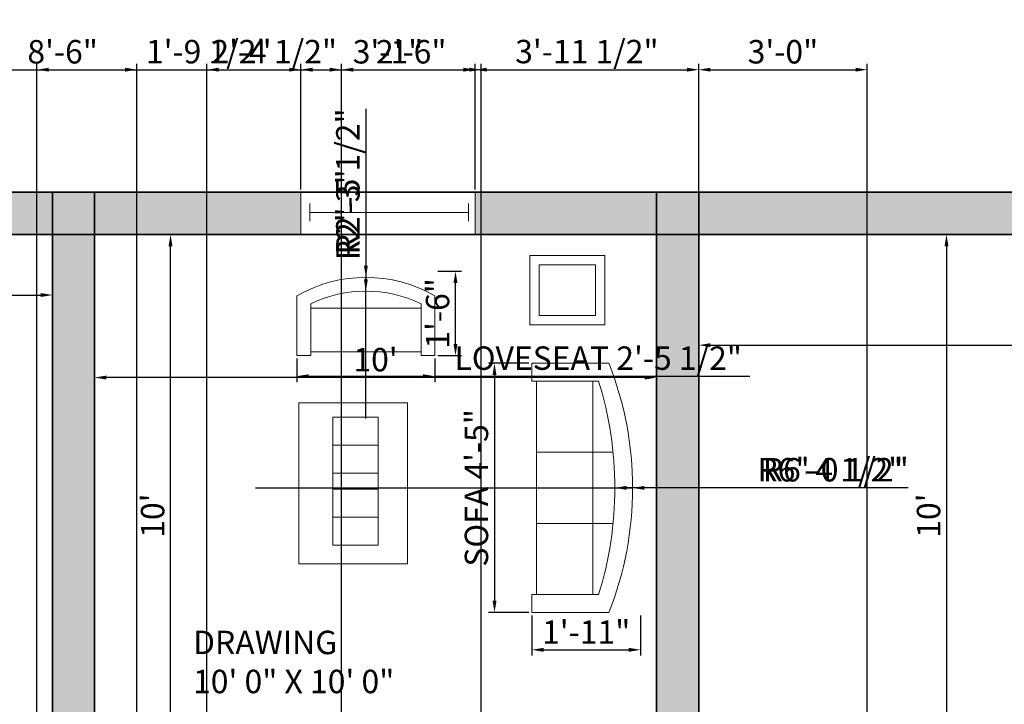
# Model space of a CAD drawing. Units: millimetres. Extents: x 2803 to 3393, y 965 to 1464.
# Tile 5 of 6: x 2962 to 3172, y 1318 to 1464. Entities that reach past the tile are written whole.
import ezdxf

# ---------------------------------------------------------------- set-up
doc = ezdxf.new("R2010")
doc.units = ezdxf.units.MM
for name, color, linetype, lineweight in [('A-ANNO-DIMS', 150, 'Continuous', 18), ('A-AREA-IDEN', 200, 'Continuous', 25), ('A-WALL-PATT', 2, 'Continuous', 13), ('furniture', 70, 'Continuous', 18), ('walls', 2, 'Continuous', 35), ('windows', 30, 'Continuous', 20)]:
    doc.layers.add(name, color=color, linetype=linetype, lineweight=lineweight)
doc.styles.get("Standard").update_dxf_attribs({"font": 'arial.ttf'})
doc.dimstyles.new('ISO-25', dxfattribs={"dimtxt": 5, "dimasz": 2.5, "dimexe": 1.25, "dimexo": 0.625, "dimtad": 1, "dimdec": 0, "dimlunit": 3, "dimtxsty": 'Standard', "dimcen": 2.5, "dimadec": 0, "dimazin": 0, "dimtfac": 1, "dimtdec": 0, "dimtmove": 0, "dimatfit": 3, "dimfxl": 1, "dimarcsym": 0})

# ---------------------------------------------------------------- blocks, each defined once
blk = doc.blocks.new('*U6')
for p, q in [((0, 4), (0, 0)), ((36, 4), (36, 0)), ((0, 2), (36, 2))]:
    blk.add_line(p, q)
blk = doc.blocks.new('Sofa - Roundback 7 ft.')
for p, q in [((-12.00002, -32.4421), (-12.00003, -6.5971)), ((11.99997, -32.4421), (11.99998, -6.5971)), ((-36.000027, -34), (-36.000027, -11.4696)), ((35.99998, -34), (35.99998, -11.4696)), ((-35.999844, -13.3819), (35.9998, -13.3819)), ((-36.000027, -32.4421), (35.99998, -32.4421))]:
    blk.add_line(p, q)
for points in [[(-36.000027, -34), (-42.000027, -34), (-42.000027, -8)], [(41.99998, -8), (41.99998, -34), (35.99998, -34)]]:
    blk.add_lwpolyline(points)
for centre, radius, start, end in [((0, -114.25), 114.25, 68.43141, 111.5686), ((-0.00001, -127.1968), 121.1968, 72.72033, 107.2797)]:
    blk.add_arc(centre, radius, start, end)
blk = doc.blocks.new('Sofa - Roundback Loveseat 5 ft.')
for p, q in [((0, -32.44198), (0, -5.99998)), ((-24, -33.99998), (-24, -11.46958)), ((24.00004, -33.99998), (24.00004, -11.46958)), ((-23.9998, -13.38178), (23.99986, -13.38178)), ((-24, -32.44198), (24.00004, -32.44198))]:
    blk.add_line(p, q)
for points in [[(-24, -33.99998), (-30, -33.99998), (-30, -7.99998)], [(30.00004, -7.99998), (30.00004, -33.99998), (24.00004, -33.99998)]]:
    blk.add_lwpolyline(points)
for centre, radius, start, end in [((0, -60.24998), 60.24998, 60.13715, 119.8628), ((0, -61.38438), 55.38444, 64.32083, 115.6792)]:
    blk.add_arc(centre, radius, start, end)
blk = doc.blocks.new('*D13')
at = {"layer": 'A-ANNO-DIMS', "color": 0, "lineweight": -2, "transparency": 16777216}
for p, q in [((2848.68, 1407.09), (2848.68, 1404.39)), ((2968.68, 1407.09), (2968.68, 1404.39)), ((2851.18, 1405.64), (2966.18, 1405.64))]:
    blk.add_line(p, q, dxfattribs=at)
at = {"layer": 'A-ANNO-DIMS', "color": 0, "transparency": 16777216}
for points in [[(2851.18, 1406.06), (2851.18, 1405.22), (2848.68, 1405.64)], [(2966.18, 1406.06), (2966.18, 1405.22), (2968.68, 1405.64)]]:
    blk.add_solid(points, dxfattribs=at)
at = {"layer": 'Defpoints', "color": 0, "transparency": 16777216}
for p in [(2848.68, 1407.71), (2968.68, 1407.71), (2968.68, 1405.64)]:
    blk.add_point(p, dxfattribs=at)
at = {"layer": 'A-ANNO-DIMS', "color": 0, "transparency": 16777216, "insert": (2908.68, 1408.82), "char_height": 5, "attachment_point": 5}
blk.add_mtext("10'", dxfattribs=at)
blk = doc.blocks.new('*D14')
at = {"layer": 'A-ANNO-DIMS', "color": 0, "lineweight": -2, "transparency": 16777216}
for p, q in [((2977.68, 1395.24), (2977.68, 1386.77)), ((3097.68, 1395.24), (3097.68, 1386.77)), ((3095.18, 1388.02), (2980.18, 1388.02))]:
    blk.add_line(p, q, dxfattribs=at)
at = {"layer": 'A-ANNO-DIMS', "color": 0, "transparency": 16777216}
for points in [[(2980.18, 1388.44), (2980.18, 1387.61), (2977.68, 1388.02)], [(3095.18, 1388.44), (3095.18, 1387.61), (3097.68, 1388.02)]]:
    blk.add_solid(points, dxfattribs=at)
at = {"layer": 'Defpoints', "color": 0, "transparency": 16777216}
for p in [(2977.68, 1395.87), (3097.68, 1395.87), (2977.68, 1388.02)]:
    blk.add_point(p, dxfattribs=at)
at = {"layer": 'A-ANNO-DIMS', "color": 0, "transparency": 16777216, "insert": (3037.68, 1391.2), "char_height": 5, "attachment_point": 5}
blk.add_mtext("10'", dxfattribs=at)
blk = doc.blocks.new('*D15')
at = {"layer": 'A-ANNO-DIMS', "color": 0, "lineweight": -2, "transparency": 16777216}
for p, q in [((2986.56, 1418.56), (2995.15, 1418.56)), ((2993.9, 1301.06), (2993.9, 1416.06)), ((2986.56, 1298.56), (2995.15, 1298.56))]:
    blk.add_line(p, q, dxfattribs=at)
at = {"layer": 'A-ANNO-DIMS', "color": 0, "transparency": 16777216}
for points in [[(2993.48, 1416.06), (2994.31, 1416.06), (2993.9, 1418.56)], [(2993.48, 1301.06), (2994.31, 1301.06), (2993.9, 1298.56)]]:
    blk.add_solid(points, dxfattribs=at)
at = {"layer": 'Defpoints', "color": 0, "transparency": 16777216}
for p in [(2985.93, 1418.56), (2993.9, 1418.56), (2985.93, 1298.56)]:
    blk.add_point(p, dxfattribs=at)
at = {"layer": 'A-ANNO-DIMS', "color": 0, "transparency": 16777216, "insert": (2990.72, 1358.56), "char_height": 5, "attachment_point": 5, "rotation": 90}
blk.add_mtext("10'", dxfattribs=at)
blk = doc.blocks.new('*D16')
at = {"layer": 'A-ANNO-DIMS', "color": 0, "lineweight": -2, "transparency": 16777216}
for p, q in [((3165.42, 1418.56), (3158.35, 1418.56)), ((3159.6, 1416.06), (3159.6, 1301.06)), ((3165.42, 1298.56), (3158.35, 1298.56))]:
    blk.add_line(p, q, dxfattribs=at)
at = {"layer": 'A-ANNO-DIMS', "color": 0, "transparency": 16777216}
for points in [[(3159.18, 1416.06), (3160.01, 1416.06), (3159.6, 1418.56)], [(3159.18, 1301.06), (3160.01, 1301.06), (3159.6, 1298.56)]]:
    blk.add_solid(points, dxfattribs=at)
at = {"layer": 'Defpoints', "color": 0, "transparency": 16777216}
for p in [(3166.04, 1418.56), (3159.6, 1298.56), (3166.04, 1298.56)]:
    blk.add_point(p, dxfattribs=at)
at = {"layer": 'A-ANNO-DIMS', "color": 0, "transparency": 16777216, "insert": (3156.42, 1358.56), "char_height": 5, "attachment_point": 5, "rotation": 90}
blk.add_mtext("10'", dxfattribs=at)
blk = doc.blocks.new('*D17')
at = {"layer": 'A-ANNO-DIMS', "color": 0, "lineweight": -2, "transparency": 16777216}
for p, q in [((3106.68, 1401.99), (3106.68, 1393.69)), ((3353.68, 1401.99), (3353.68, 1393.69)), ((3109.18, 1394.94), (3351.18, 1394.94))]:
    blk.add_line(p, q, dxfattribs=at)
at = {"layer": 'A-ANNO-DIMS', "color": 0, "transparency": 16777216}
for points in [[(3109.18, 1395.36), (3109.18, 1394.53), (3106.68, 1394.94)], [(3351.18, 1395.36), (3351.18, 1394.53), (3353.68, 1394.94)]]:
    blk.add_solid(points, dxfattribs=at)
at = {"layer": 'Defpoints', "color": 0, "transparency": 16777216}
for p in [(3106.68, 1402.61), (3353.68, 1402.61), (3353.68, 1394.94)]:
    blk.add_point(p, dxfattribs=at)
at = {"layer": 'A-ANNO-DIMS', "color": 0, "transparency": 16777216, "insert": (3230.18, 1398.12), "char_height": 5, "attachment_point": 5}
blk.add_mtext('20\'-7"', dxfattribs=at)
blk = doc.blocks.new('*D35')
at = {"layer": 'A-ANNO-DIMS', "color": 0, "lineweight": -2, "transparency": 16777216}
for p, q in [((3070.43, 1391.07), (3061.83, 1391.07)), ((3063.08, 1388.57), (3063.08, 1340.4)), ((3070.43, 1337.9), (3061.83, 1337.9))]:
    blk.add_line(p, q, dxfattribs=at)
at = {"layer": 'A-ANNO-DIMS', "color": 0, "transparency": 16777216}
for points in [[(3062.67, 1388.57), (3063.5, 1388.57), (3063.08, 1391.07)], [(3062.67, 1340.4), (3063.5, 1340.4), (3063.08, 1337.9)]]:
    blk.add_solid(points, dxfattribs=at)
at = {"layer": 'Defpoints', "color": 0, "transparency": 16777216}
for p in [(3071.06, 1391.07), (3063.08, 1337.9), (3071.06, 1337.9)]:
    blk.add_point(p, dxfattribs=at)
at = {"layer": 'A-ANNO-DIMS', "color": 0, "transparency": 16777216, "insert": (3059.87, 1364.49), "char_height": 5, "attachment_point": 5, "rotation": 90}
blk.add_mtext('SOFA 4\'-5"', dxfattribs=at)
blk = doc.blocks.new('*D36')
at = {"layer": 'A-ANNO-DIMS', "color": 0, "lineweight": -2, "transparency": 16777216}
for p, q in [((3071.06, 1337.28), (3071.06, 1328.68)), ((3094.26, 1337.28), (3094.26, 1328.68)), ((3073.56, 1329.93), (3091.76, 1329.93))]:
    blk.add_line(p, q, dxfattribs=at)
at = {"layer": 'A-ANNO-DIMS', "color": 0, "transparency": 16777216}
for points in [[(3073.56, 1330.34), (3073.56, 1329.51), (3071.06, 1329.93)], [(3091.76, 1330.34), (3091.76, 1329.51), (3094.26, 1329.93)]]:
    blk.add_solid(points, dxfattribs=at)
at = {"layer": 'Defpoints', "color": 0, "transparency": 16777216}
for p in [(3071.06, 1337.9), (3094.26, 1337.9), (3094.26, 1329.93)]:
    blk.add_point(p, dxfattribs=at)
at = {"layer": 'A-ANNO-DIMS', "color": 0, "transparency": 16777216, "insert": (3082.66, 1333.06), "char_height": 5, "attachment_point": 5}
blk.add_mtext('1\'-11"', dxfattribs=at)
blk = doc.blocks.new('*D37')
at = {"layer": 'A-ANNO-DIMS', "color": 0, "lineweight": -2, "transparency": 16777216}
for p, q in [((3020.89, 1392.1), (3020.89, 1387.05)), ((3050.34, 1392.1), (3050.34, 1387.05)), ((3023.39, 1388.3), (3047.84, 1388.3)), ((3050.34, 1388.3), (3117.63, 1388.3))]:
    blk.add_line(p, q, dxfattribs=at)
at = {"layer": 'A-ANNO-DIMS', "color": 0, "transparency": 16777216}
for points in [[(3023.39, 1388.72), (3023.39, 1387.89), (3020.89, 1388.3)], [(3047.84, 1388.72), (3047.84, 1387.89), (3050.34, 1388.3)]]:
    blk.add_solid(points, dxfattribs=at)
at = {"layer": 'Defpoints', "color": 0, "transparency": 16777216}
for p in [(3020.89, 1392.72), (3050.34, 1392.72), (3050.34, 1388.3)]:
    blk.add_point(p, dxfattribs=at)
at = {"layer": 'A-ANNO-DIMS', "color": 0, "transparency": 16777216, "insert": (3085.23, 1391.52), "char_height": 5, "attachment_point": 5}
blk.add_mtext('LOVESEAT 2\'-5 1/2"', dxfattribs=at)
blk = doc.blocks.new('*D38')
at = {"layer": 'A-ANNO-DIMS', "color": 0, "lineweight": -2, "transparency": 16777216}
for p, q in [((3050.96, 1410.71), (3056, 1410.71)), ((3054.75, 1395.22), (3054.75, 1408.21)), ((3050.96, 1392.72), (3056, 1392.72))]:
    blk.add_line(p, q, dxfattribs=at)
at = {"layer": 'A-ANNO-DIMS', "color": 0, "transparency": 16777216}
for points in [[(3054.33, 1408.21), (3055.17, 1408.21), (3054.75, 1410.71)], [(3054.33, 1395.22), (3055.17, 1395.22), (3054.75, 1392.72)]]:
    blk.add_solid(points, dxfattribs=at)
at = {"layer": 'Defpoints', "color": 0, "transparency": 16777216}
for p in [(3050.34, 1410.71), (3054.75, 1410.71), (3050.34, 1392.72)]:
    blk.add_point(p, dxfattribs=at)
at = {"layer": 'A-ANNO-DIMS', "color": 0, "transparency": 16777216, "insert": (3051.57, 1401.72), "char_height": 5, "attachment_point": 5, "rotation": 90}
blk.add_mtext('1\'-6"', dxfattribs=at)
blk = doc.blocks.new('*D43')
at = {"layer": 'A-ANNO-DIMS', "color": 0, "lineweight": -2, "transparency": 16777216}
for p, q in [((3106.68, 1230.24), (3106.68, 1454.97)), ((3109.18, 1453.72), (3140.18, 1453.72)), ((3142.68, 1230.24), (3142.68, 1454.97))]:
    blk.add_line(p, q, dxfattribs=at)
at = {"layer": 'A-ANNO-DIMS', "color": 0, "transparency": 16777216}
for points in [[(3109.18, 1454.14), (3109.18, 1453.31), (3106.68, 1453.72)], [(3140.18, 1454.14), (3140.18, 1453.31), (3142.68, 1453.72)]]:
    blk.add_solid(points, dxfattribs=at)
at = {"layer": 'Defpoints', "color": 0, "transparency": 16777216}
for p in [(3142.68, 1453.72), (3106.68, 1229.61), (3142.68, 1229.61)]:
    blk.add_point(p, dxfattribs=at)
at = {"layer": 'A-ANNO-DIMS', "color": 0, "transparency": 16777216, "insert": (3124.68, 1456.9), "char_height": 5, "attachment_point": 5}
blk.add_mtext('3\'-0"', dxfattribs=at)
blk = doc.blocks.new('*D51')
at = {"layer": 'A-ANNO-DIMS', "color": 0, "lineweight": -2, "transparency": 16777216}
for p, q in [((2919.98, 1428.19), (2919.98, 1454.97)), ((2922.48, 1453.72), (3019.24, 1453.72)), ((3021.74, 1428.19), (3021.74, 1454.97))]:
    blk.add_line(p, q, dxfattribs=at)
at = {"layer": 'A-ANNO-DIMS', "color": 0, "transparency": 16777216}
for points in [[(2922.48, 1454.14), (2922.48, 1453.31), (2919.98, 1453.72)], [(3019.24, 1454.14), (3019.24, 1453.31), (3021.74, 1453.72)]]:
    blk.add_solid(points, dxfattribs=at)
at = {"layer": 'Defpoints', "color": 0, "transparency": 16777216}
for p in [(3021.74, 1453.72), (2919.98, 1427.56), (3021.74, 1427.56)]:
    blk.add_point(p, dxfattribs=at)
at = {"layer": 'A-ANNO-DIMS', "color": 0, "transparency": 16777216, "insert": (2970.86, 1456.9), "char_height": 5, "attachment_point": 5}
blk.add_mtext('8\'-6"', dxfattribs=at)
blk = doc.blocks.new('*D52')
at = {"layer": 'A-ANNO-DIMS', "color": 0, "lineweight": -2, "transparency": 16777216}
for p, q in [((3021.74, 1428.19), (3021.74, 1454.97)), ((3024.24, 1453.72), (3056.44, 1453.72)), ((3058.94, 1428.19), (3058.94, 1454.97))]:
    blk.add_line(p, q, dxfattribs=at)
at = {"layer": 'A-ANNO-DIMS', "color": 0, "transparency": 16777216}
for points in [[(3024.24, 1454.14), (3024.24, 1453.31), (3021.74, 1453.72)], [(3056.44, 1454.14), (3056.44, 1453.31), (3058.94, 1453.72)]]:
    blk.add_solid(points, dxfattribs=at)
at = {"layer": 'Defpoints', "color": 0, "transparency": 16777216}
for p in [(3058.94, 1453.72), (3021.74, 1427.56), (3058.94, 1427.56)]:
    blk.add_point(p, dxfattribs=at)
at = {"layer": 'A-ANNO-DIMS', "color": 0, "transparency": 16777216, "insert": (3040.34, 1456.9), "char_height": 5, "attachment_point": 5}
blk.add_mtext('3\'-1"', dxfattribs=at)
blk = doc.blocks.new('*D53')
at = {"layer": 'A-ANNO-DIMS', "color": 0, "lineweight": -2, "transparency": 16777216}
for p, q in [((3058.94, 1428.19), (3058.94, 1454.97)), ((3061.44, 1453.72), (3104.18, 1453.72)), ((3106.68, 1428.19), (3106.68, 1454.97))]:
    blk.add_line(p, q, dxfattribs=at)
at = {"layer": 'A-ANNO-DIMS', "color": 0, "transparency": 16777216}
for points in [[(3061.44, 1454.14), (3061.44, 1453.31), (3058.94, 1453.72)], [(3104.18, 1454.14), (3104.18, 1453.31), (3106.68, 1453.72)]]:
    blk.add_solid(points, dxfattribs=at)
at = {"layer": 'Defpoints', "color": 0, "transparency": 16777216}
for p in [(3106.68, 1453.72), (3058.94, 1427.56), (3106.68, 1427.56)]:
    blk.add_point(p, dxfattribs=at)
at = {"layer": 'A-ANNO-DIMS', "color": 0, "transparency": 16777216, "insert": (3082.81, 1456.94), "char_height": 5, "attachment_point": 5}
blk.add_mtext('3\'-11 1/2"', dxfattribs=at)
blk = doc.blocks.new('*D61')
at = {"layer": 'A-ANNO-DIMS', "color": 0, "lineweight": -2, "transparency": 16777216}
for p, q in [((3001.68, 1025.19), (3001.68, 1454.97)), ((3004.18, 1453.72), (3027.9, 1453.72)), ((3030.4, 1025.19), (3030.4, 1454.97))]:
    blk.add_line(p, q, dxfattribs=at)
at = {"layer": 'A-ANNO-DIMS', "color": 0, "transparency": 16777216}
for points in [[(3004.18, 1454.14), (3004.18, 1453.31), (3001.68, 1453.72)], [(3027.9, 1454.14), (3027.9, 1453.31), (3030.4, 1453.72)]]:
    blk.add_solid(points, dxfattribs=at)
at = {"layer": 'Defpoints', "color": 0, "transparency": 16777216}
for p in [(3030.4, 1453.72), (3001.68, 1024.56), (3030.4, 1024.56)]:
    blk.add_point(p, dxfattribs=at)
at = {"layer": 'A-ANNO-DIMS', "color": 0, "transparency": 16777216, "insert": (3016.04, 1456.93), "char_height": 5, "attachment_point": 5}
blk.add_mtext('2\'-4 1/2"', dxfattribs=at)
blk = doc.blocks.new('*D62')
at = {"layer": 'A-ANNO-DIMS', "color": 0, "lineweight": -2, "transparency": 16777216}
for p, q in [((3030.4, 1025.19), (3030.4, 1454.97)), ((3032.9, 1453.72), (3057.7, 1453.72)), ((3060.2, 1025.19), (3060.2, 1454.97))]:
    blk.add_line(p, q, dxfattribs=at)
at = {"layer": 'A-ANNO-DIMS', "color": 0, "transparency": 16777216}
for points in [[(3032.9, 1454.14), (3032.9, 1453.31), (3030.4, 1453.72)], [(3057.7, 1454.14), (3057.7, 1453.31), (3060.2, 1453.72)]]:
    blk.add_solid(points, dxfattribs=at)
at = {"layer": 'Defpoints', "color": 0, "transparency": 16777216}
for p in [(3060.2, 1453.72), (3030.4, 1024.56), (3060.2, 1024.56)]:
    blk.add_point(p, dxfattribs=at)
at = {"layer": 'A-ANNO-DIMS', "color": 0, "transparency": 16777216, "insert": (3045.3, 1456.9), "char_height": 5, "attachment_point": 5}
blk.add_mtext('2\'-6"', dxfattribs=at)
blk = doc.blocks.new('*D63')
at = {"layer": 'A-ANNO-DIMS', "color": 0, "lineweight": -2, "transparency": 16777216}
for p, q in [((2968.68, 1426.94), (2968.68, 968.15)), ((2977.68, 1426.94), (2977.68, 968.15)), ((2971.18, 969.4), (2975.18, 969.4)), ((2977.68, 969.4), (2994.73, 969.4))]:
    blk.add_line(p, q, dxfattribs=at)
at = {"layer": 'A-ANNO-DIMS', "color": 0, "transparency": 16777216}
for points in [[(2971.18, 969.82), (2971.18, 968.99), (2968.68, 969.4)], [(2975.18, 969.82), (2975.18, 968.99), (2977.68, 969.4)]]:
    blk.add_solid(points, dxfattribs=at)
at = {"layer": 'Defpoints', "color": 0, "transparency": 16777216}
for p in [(2968.68, 1427.56), (2977.68, 1427.56), (2977.68, 969.4)]:
    blk.add_point(p, dxfattribs=at)
at = {"layer": 'A-ANNO-DIMS', "color": 0, "transparency": 16777216, "insert": (2987.45, 972.58), "char_height": 5, "attachment_point": 5}
blk.add_mtext('0\'-9"', dxfattribs=at)
blk = doc.blocks.new('*D70')
at = {"layer": 'A-ANNO-DIMS', "color": 0, "lineweight": -2, "transparency": 16777216}
for p, q in [((2965.38, 1175.19), (2965.38, 1454.97)), ((2967.88, 1453.72), (2984.19, 1453.72)), ((2986.69, 1175.19), (2986.69, 1454.97)), ((2986.69, 1453.72), (3014.92, 1453.72))]:
    blk.add_line(p, q, dxfattribs=at)
at = {"layer": 'A-ANNO-DIMS', "color": 0, "transparency": 16777216}
for points in [[(2967.88, 1454.14), (2967.88, 1453.31), (2965.38, 1453.72)], [(2984.19, 1454.14), (2984.19, 1453.31), (2986.69, 1453.72)]]:
    blk.add_solid(points, dxfattribs=at)
at = {"layer": 'Defpoints', "color": 0, "transparency": 16777216}
for p in [(2986.69, 1453.72), (2965.38, 1174.56), (2986.69, 1174.56)]:
    blk.add_point(p, dxfattribs=at)
at = {"layer": 'A-ANNO-DIMS', "color": 0, "transparency": 16777216, "insert": (3002.06, 1456.93), "char_height": 5, "attachment_point": 5}
blk.add_mtext('1\'-9 1/2"', dxfattribs=at)
blk = doc.blocks.new('*D75')
at = {"layer": 'A-ANNO-DIMS', "color": 0, "lineweight": -2, "transparency": 16777216}
for p, q in [((3012.07, 1364.48), (3088.78, 1364.48)), ((3150.29, 1364.48), (3091.28, 1364.48))]:
    blk.add_line(p, q, dxfattribs=at)
at = {"layer": 'A-ANNO-DIMS', "color": 0, "transparency": 16777216}
blk.add_solid([(3091.28, 1364.9), (3091.28, 1364.07), (3088.78, 1364.48)], dxfattribs=at)
at = {"layer": 'Defpoints', "color": 0, "transparency": 16777216}
for p in [(3012.07, 1364.48), (3088.78, 1364.48)]:
    blk.add_point(p, dxfattribs=at)
at = {"layer": 'A-ANNO-DIMS', "color": 0, "transparency": 16777216, "insert": (3134.8, 1367.7), "char_height": 5, "attachment_point": 5, "rotation": 360}
blk.add_mtext('R6\'-4 1/2"', dxfattribs=at)
blk = doc.blocks.new('*D76')
at = {"layer": 'A-ANNO-DIMS', "color": 0, "lineweight": -2, "transparency": 16777216}
for p, q in [((3020.27, 1364.48), (3092.58, 1364.48)), ((3151.45, 1364.48), (3095.08, 1364.48))]:
    blk.add_line(p, q, dxfattribs=at)
at = {"layer": 'A-ANNO-DIMS', "color": 0, "transparency": 16777216}
blk.add_solid([(3095.08, 1364.9), (3095.08, 1364.07), (3092.58, 1364.48)], dxfattribs=at)
at = {"layer": 'Defpoints', "color": 0, "transparency": 16777216}
for p in [(3020.27, 1364.48), (3092.58, 1364.48)]:
    blk.add_point(p, dxfattribs=at)
at = {"layer": 'A-ANNO-DIMS', "color": 0, "transparency": 16777216, "insert": (3135.96, 1367.7), "char_height": 5, "attachment_point": 5, "rotation": 360}
blk.add_mtext('R6\'-0 1/2"', dxfattribs=at)
blk = doc.blocks.new('*D77')
at = {"layer": 'A-ANNO-DIMS', "color": 0, "lineweight": -2, "transparency": 16777216}
for p, q in [((3035.61, 1445.38), (3035.61, 1411.9)), ((3035.61, 1379.84), (3035.61, 1409.4))]:
    blk.add_line(p, q, dxfattribs=at)
at = {"layer": 'A-ANNO-DIMS', "color": 0, "transparency": 16777216}
blk.add_solid([(3035.2, 1411.9), (3036.03, 1411.9), (3035.61, 1409.4)], dxfattribs=at)
at = {"layer": 'Defpoints', "color": 0, "transparency": 16777216}
for p in [(3035.61, 1409.4), (3035.61, 1379.84)]:
    blk.add_point(p, dxfattribs=at)
at = {"layer": 'A-ANNO-DIMS', "color": 0, "transparency": 16777216, "insert": (3032.4, 1429.89), "char_height": 5, "attachment_point": 5, "rotation": 89.9999}
blk.add_mtext('R2\'-5 1/2"', dxfattribs=at)
blk = doc.blocks.new('*D78')
at = {"layer": 'A-ANNO-DIMS', "color": 0, "lineweight": -2, "transparency": 16777216}
for p, q in [((3035.61, 1432.43), (3035.61, 1408.96)), ((3035.61, 1379.28), (3035.61, 1406.46))]:
    blk.add_line(p, q, dxfattribs=at)
at = {"layer": 'A-ANNO-DIMS', "color": 0, "transparency": 16777216}
blk.add_solid([(3035.2, 1408.96), (3036.03, 1408.96), (3035.61, 1406.46)], dxfattribs=at)
at = {"layer": 'Defpoints', "color": 0, "transparency": 16777216}
for p in [(3035.61, 1406.46), (3035.61, 1379.28)]:
    blk.add_point(p, dxfattribs=at)
at = {"layer": 'A-ANNO-DIMS', "color": 0, "transparency": 16777216, "insert": (3032.44, 1422.76), "char_height": 5, "attachment_point": 5, "rotation": 89.9999}
blk.add_mtext('R2\'-3"', dxfattribs=at)

msp = doc.modelspace()

# ---------------------------------------------------------------- hatches: boundary and pattern name
at = {"layer": 'A-WALL-PATT'}
h = msp.add_hatch(color=256, dxfattribs=at)
h.dxf.hatch_style = 1
h.paths.add_polyline_path([(2968.68, 1427.56), (2919.98, 1427.56), (2919.98, 1418.56), (2968.68, 1418.56)])
h.paths.add_polyline_path([(2977.68, 1427.56), (2968.68, 1427.56), (2968.68, 1418.56), (2977.68, 1418.56)])
h.paths.add_polyline_path([(2977.68, 1418.56), (2968.68, 1418.56), (2968.68, 1298.56), (2977.68, 1298.56)])
h.paths.add_polyline_path([(3021.74, 1427.56), (2977.68, 1427.56), (2977.68, 1418.56), (3021.74, 1418.56)])
h.paths.add_polyline_path([(2881.7, 1427.56), (2848.68, 1427.56), (2848.68, 1418.56), (2881.7, 1418.56)])
h.paths.add_polyline_path([(2848.68, 1427.56), (2839.68, 1427.56), (2839.68, 1418.56), (2848.68, 1418.56)])
h.paths.add_polyline_path([(2848.68, 1418.56), (2839.68, 1418.56), (2839.68, 1298.56), (2848.68, 1298.56)])
h.paths.add_polyline_path([(2932.68, 1298.56), (2848.68, 1298.56), (2848.68, 1289.56), (2932.68, 1289.56)])
h.paths.add_polyline_path([(2848.68, 1298.56), (2839.68, 1298.56), (2839.68, 1289.56), (2848.68, 1289.56)])
h.paths.add_polyline_path([(2848.68, 1289.56), (2839.68, 1289.56), (2839.68, 1280.88), (2848.68, 1280.88)])
h.paths.add_polyline_path([(2848.68, 1252.94), (2839.68, 1252.94), (2839.68, 1241.56), (2848.68, 1241.56)])
h.paths.add_polyline_path([(2848.68, 1241.56), (2839.68, 1241.56), (2839.68, 1232.56), (2848.68, 1232.56)])
h.paths.add_polyline_path([(2932.68, 1241.56), (2848.68, 1241.56), (2848.68, 1232.56), (2932.68, 1232.56)])
h.paths.add_polyline_path([(2941.68, 1241.56), (2932.68, 1241.56), (2932.68, 1232.56), (2941.68, 1232.56)])
h.paths.add_polyline_path([(2941.68, 1289.56), (2932.68, 1289.56), (2932.68, 1257.22, -0.114666), (2939.92, 1259.03), (2941.68, 1259.07)])
h.paths.add_polyline_path([(2941.68, 1298.56), (2932.68, 1298.56), (2932.68, 1289.56), (2941.68, 1289.56)])
h.paths.add_polyline_path([(2947.42, 1298.56), (2941.68, 1298.56), (2941.68, 1289.56), (2945.75, 1289.56), (2945.75, 1290.29, -0.099582)])
h.paths.add_polyline_path([(2977.68, 1298.56), (2968.68, 1298.56), (2968.68, 1289.56), (2977.68, 1289.56)])
h.paths.add_polyline_path([(3018.47, 1298.56), (2977.68, 1298.56), (2977.68, 1289.56), (3018.47, 1289.56)])
h.paths.add_polyline_path([(3097.68, 1298.56), (3067.31, 1298.56), (3067.31, 1289.56), (3097.68, 1289.56)])
h.paths.add_polyline_path([(3106.68, 1298.56), (3097.68, 1298.56), (3097.68, 1289.56), (3106.68, 1289.56)])
h.paths.add_polyline_path([(3200.68, 1298.56), (3106.68, 1298.56), (3106.68, 1289.56), (3200.68, 1289.56)])
h.paths.add_polyline_path([(3209.68, 1298.56), (3200.68, 1298.56), (3200.68, 1289.56), (3209.68, 1289.56)])
h.paths.add_polyline_path([(3209.68, 1289.56), (3200.68, 1289.56), (3200.68, 1270.22), (3209.68, 1270.22)])
h.paths.add_polyline_path([(3106.68, 1418.56), (3097.68, 1418.56), (3097.68, 1298.56), (3106.68, 1298.56)])
h.paths.add_polyline_path([(3106.68, 1427.56), (3097.68, 1427.56), (3097.68, 1418.56), (3106.68, 1418.56)])
h.paths.add_polyline_path([(3097.68, 1427.56), (3058.94, 1427.56), (3058.94, 1418.56), (3097.68, 1418.56)])
h.paths.add_polyline_path([(3353.68, 1427.56), (3106.68, 1427.56), (3106.68, 1418.56), (3353.68, 1418.56)])
h.paths.add_polyline_path([(3362.68, 1427.56), (3353.68, 1427.56), (3353.68, 1418.56), (3362.68, 1418.56)])
h.paths.add_polyline_path([(3362.68, 1418.56), (3353.68, 1418.56), (3353.68, 1064.56), (3362.68, 1064.56)])
h.paths.add_polyline_path([(3362.68, 1064.56), (3353.68, 1064.56), (3353.68, 1055.56), (3362.68, 1055.56)])
h.paths.add_polyline_path([(3362.68, 1055.56), (3353.68, 1055.56), (3353.68, 995.56), (3362.68, 995.56)])
h.paths.add_polyline_path([(3353.68, 1064.56), (3209.68, 1064.56), (3209.68, 1055.56), (3353.68, 1055.56)])
h.paths.add_polyline_path([(3200.68, 1064.56), (3106.68, 1064.56), (3106.68, 1055.56), (3200.68, 1055.56)])
h.paths.add_polyline_path([(3209.68, 1064.56), (3200.68, 1064.56), (3200.68, 1055.56), (3209.68, 1055.56)])
h.paths.add_polyline_path([(3209.68, 1229.61), (3200.68, 1229.61), (3200.68, 1064.56), (3209.68, 1064.56)])
h.paths.add_polyline_path([(3106.68, 1117.56), (3097.68, 1117.56), (3097.68, 1064.56), (3106.68, 1064.56)])
h.paths.add_polyline_path([(3106.68, 1126.56), (3097.68, 1126.56), (3097.68, 1117.56), (3106.68, 1117.56)])
h.paths.add_polyline_path([(3097.68, 1126.56), (3001.68, 1126.56), (3001.68, 1117.56), (3097.68, 1117.56)])
h.paths.add_polyline_path([(3001.68, 1165.56), (2992.68, 1165.56), (2992.68, 1126.56), (3001.68, 1126.56)])
h.paths.add_polyline_path([(3001.68, 1174.56), (2992.68, 1174.56), (2992.68, 1165.56), (3001.68, 1165.56)])
h.paths.add_polyline_path([(2992.68, 1174.56), (2986.69, 1174.56), (2986.69, 1165.56), (2992.68, 1165.56)])
h.paths.add_polyline_path([(3001.68, 1126.56), (2992.68, 1126.56), (2992.68, 1117.56), (3001.68, 1117.56)])
h.paths.add_polyline_path([(3001.68, 1117.56), (2992.68, 1117.56), (2992.68, 1112.21), (2994.15, 1112.23), (3001.68, 1112.37)])
h.paths.add_polyline_path([(3001.68, 1033.56), (2992.68, 1033.56), (2992.68, 1024.56), (3001.68, 1024.56)])
h.paths.add_polyline_path([(3001.68, 1097.58, -0.114732), (2994.45, 1095.76), (2992.68, 1095.73), (2992.68, 1033.56), (3001.68, 1033.56)])
h.paths.add_polyline_path([(3030.4, 1033.56), (3001.68, 1033.56), (3001.68, 1024.56), (3030.4, 1024.56)])
h.paths.add_polyline_path([(3097.68, 1033.56), (3060.2, 1033.56), (3060.2, 1024.56), (3097.68, 1024.56)])
h.paths.add_polyline_path([(3106.68, 1033.56), (3097.68, 1033.56), (3097.68, 1024.56), (3106.68, 1024.56)])
h.paths.add_polyline_path([(3106.68, 1055.56), (3097.68, 1055.56), (3097.68, 1033.56), (3106.68, 1033.56)])
h.paths.add_polyline_path([(3106.68, 1064.56), (3097.68, 1064.56), (3097.68, 1055.56), (3106.68, 1055.56)])
h.paths.add_polyline_path([(2992.68, 1033.56), (2848.68, 1033.56), (2848.68, 1024.56), (2992.68, 1024.56)])
h.paths.add_polyline_path([(2848.68, 1033.56), (2839.68, 1033.56), (2839.68, 1024.56), (2848.68, 1024.56)])
h.paths.add_polyline_path([(2848.68, 1070.54), (2839.68, 1070.54), (2839.68, 1033.56), (2848.68, 1033.56)])
h.paths.add_polyline_path([(2848.68, 1165.56), (2839.68, 1165.56), (2839.68, 1114.52), (2848.68, 1114.52)])
h.paths.add_polyline_path([(2848.68, 1174.56), (2839.68, 1174.56), (2839.68, 1165.56), (2848.68, 1165.56)])
h.paths.add_polyline_path([(2932.68, 1174.56), (2848.68, 1174.56), (2848.68, 1165.56), (2932.68, 1165.56)])
h.paths.add_polyline_path([(2941.68, 1174.56), (2932.68, 1174.56), (2932.68, 1165.56), (2941.68, 1165.56)])
h.paths.add_polyline_path([(2965.38, 1174.56), (2941.68, 1174.56), (2941.68, 1165.56), (2968.2, 1165.56, -0.111634)])
h.paths.add_polyline_path([(2848.68, 1193.13), (2839.68, 1193.13), (2839.68, 1174.56), (2848.68, 1174.56)])
h.paths.add_polyline_path([(2848.68, 1232.56), (2839.68, 1232.56), (2839.68, 1221.86), (2848.68, 1221.86)])
h.paths.add_polyline_path([(2941.68, 1232.56), (2932.68, 1232.56), (2932.68, 1191.24, -0.132111), (2940.91, 1193.6), (2941.68, 1193.62)])
h.paths.add_polyline_path([(3106.68, 1262.96), (3105.94, 1262.96, -0.099353), (3097.68, 1264.61), (3097.68, 1126.56), (3106.68, 1126.56)])

# ---------------------------------------------------------------- linework, layer by layer
at = {"layer": 'furniture'}
for p, q in [((3028.53, 1379.59), (3038.23, 1379.59)), ((3028.53, 1352.22), (3028.53, 1379.59)), ((3038.23, 1379.59), (3038.23, 1352.22)), ((3028.53, 1373.59), (3038.23, 1373.59)), ((3028.53, 1367.59), (3038.23, 1367.59)), ((3038.23, 1364.22), (3028.53, 1364.22)), ((3038.23, 1358.22), (3028.53, 1358.22)), ((3038.23, 1352.22), (3028.53, 1352.22))]:
    msp.add_line(p, q, dxfattribs=at)
for points in [[(3070.62, 1414.07), (3086.67, 1414.07), (3086.67, 1399.26), (3070.62, 1399.26)], [(3072.62, 1412.07), (3084.67, 1412.07), (3084.67, 1401.26), (3072.62, 1401.26)], [(3021.28, 1382.61), (3044.48, 1382.61), (3044.48, 1348.29), (3021.28, 1348.29)]]:
    msp.add_lwpolyline(points, close=True, dxfattribs=at)
at = {"layer": 'walls'}
for p, q in [((2839.68, 1427.56), (3362.68, 1427.56)), ((2968.68, 1427.56), (2968.68, 1289.56)), ((2977.68, 1427.56), (2977.68, 1289.56)), ((3097.68, 1427.56), (3097.68, 1284.35)), ((3106.68, 1427.56), (3106.68, 1284.35)), ((2839.68, 1418.56), (3362.68, 1418.56))]:
    msp.add_line(p, q, dxfattribs=at)
at = {"layer": 'windows'}
for p, q in [((3021.74, 1427.56), (3021.74, 1418.56)), ((3058.94, 1427.56), (3058.94, 1418.56))]:
    msp.add_line(p, q, dxfattribs=at)

# ---------------------------------------------------------------- block references
at = {"layer": 'furniture', "xscale": 0.4906690843823473, "yscale": 0.4906690843823473, "zscale": 0.4906690843823473}
msp.add_blockref('Sofa - Roundback Loveseat 5 ft.', (3035.61, 1409.4), dxfattribs=at)
at = {"layer": 'furniture', "xscale": 0.6329226737076415, "yscale": 0.6329226737076415, "zscale": 0.6329226737076415, "rotation": 270}
msp.add_blockref('Sofa - Roundback 7 ft.', (3092.58, 1364.48), dxfattribs=at)
at = {"layer": 'windows', "xscale": 0.9425308196764994, "yscale": 0.9425308196764994, "zscale": 0.9425308196764994}
msp.add_blockref('*U6', (3023.62, 1421.37), dxfattribs=at)

# ---------------------------------------------------------------- texts
at = {"layer": 'A-AREA-IDEN', "insert": (2998.7, 1334), "char_height": 5, "attachment_point": 1}
msp.add_mtext_dynamic_manual_height_columns('DRAWING \\P10\' 0" X 10\' 0"', width=57.2389, gutter_width=12.5, heights=[0], dxfattribs=at)

# ---------------------------------------------------------------- dimensions: what is measured, and where the dimension line sits
at = {"layer": 'A-ANNO-DIMS'}
for base, p1, p2, override, picture, middle in [((2986.69, 1453.72), (2965.38, 1174.56), (2986.69, 1174.56), {"dimdec": 1, "dimlfac": 1, "dimrnd": 0, "dimzin": 1, "dimdsep": 46, "dimlunit": 4, "dimfrac": 2}, '*D70', (3002.06, 1456.93)), ((3030.4, 1453.72), (3001.68, 1024.56), (3030.4, 1024.56), {"dimdec": 1, "dimlfac": 1, "dimrnd": 0, "dimzin": 1, "dimdsep": 46, "dimlunit": 4, "dimfrac": 2}, '*D61', (3016.04, 1456.93)), ((3106.68, 1453.72), (3058.94, 1427.56), (3106.68, 1427.56), {"dimdec": 1, "dimlfac": 1, "dimrnd": 0, "dimzin": 1, "dimdsep": 46, "dimlunit": 4, "dimfrac": 2}, '*D53', (3082.81, 1456.94)), ((3021.74, 1453.72), (2919.98, 1427.56), (3021.74, 1427.56), {"dimdec": 1, "dimlfac": 1, "dimrnd": 0, "dimzin": 1, "dimdsep": 46, "dimlunit": 4, "dimfrac": 2}, '*D51', (2970.86, 1456.9)), ((3058.94, 1453.72), (3021.74, 1427.56), (3058.94, 1427.56), {"dimdec": 1, "dimlfac": 1, "dimrnd": 0, "dimzin": 1, "dimdsep": 46, "dimlunit": 4, "dimfrac": 2}, '*D52', (3040.34, 1456.9)), ((3060.2, 1453.72), (3030.4, 1024.56), (3060.2, 1024.56), {"dimdec": 1, "dimlfac": 1, "dimrnd": 0, "dimzin": 1, "dimdsep": 46, "dimlunit": 4, "dimfrac": 2}, '*D62', (3045.3, 1456.9)), ((3142.68, 1453.72), (3106.68, 1229.61), (3142.68, 1229.61), {"dimdec": 1, "dimlfac": 1, "dimrnd": 0, "dimzin": 1, "dimdsep": 46, "dimlunit": 4, "dimfrac": 2}, '*D43', (3124.68, 1456.9)), ((2977.68, 969.4), (2968.68, 1427.56), (2977.68, 1427.56), {"dimdec": 1, "dimlfac": 1, "dimrnd": 0, "dimzin": 1, "dimdsep": 46, "dimlunit": 4, "dimfrac": 2}, '*D63', (2987.45, 972.58)), ((2968.68, 1405.64), (2848.68, 1407.71), (2968.68, 1407.71), {"dimclrd": 0, "dimclre": 0, "dimclrt": 0}, '*D13', (2908.68, 1408.82)), ((3353.68, 1394.94), (3106.68, 1402.61), (3353.68, 1402.61), {"dimclrd": 0, "dimclre": 0, "dimclrt": 0}, '*D17', (3230.18, 1398.12)), ((2977.68, 1388.02), (3097.68, 1395.87), (2977.68, 1395.87), {"dimclrd": 0, "dimclre": 0, "dimclrt": 0}, '*D14', (3037.68, 1391.2)), ((3094.26, 1329.93), (3071.06, 1337.9), (3094.26, 1337.9), {"dimdec": 1, "dimlfac": 1, "dimrnd": 0, "dimzin": 1, "dimdsep": 46, "dimlunit": 4, "dimfrac": 2}, '*D36', (3082.66, 1333.06))]:
    dim = msp.add_linear_dim(base=base, p1=p1, p2=p2, dimstyle='ISO-25', override=override, dxfattribs=at)
    dim.commit()
    dim.dimension.update_dxf_attribs({"geometry": picture, "text_midpoint": middle})
dim = msp.add_radius_dim(center=(3035.61, 1379.84), mpoint=(3035.61, 1409.4), dimstyle='ISO-25', override={"dimdec": 1, "dimlfac": 1, "dimrnd": 0, "dimzin": 1, "dimdsep": 46, "dimlunit": 4, "dimfrac": 2}, dxfattribs=at)
dim.commit()
dim.dimension.update_dxf_attribs({"geometry": '*D77', "text_midpoint": (3032.4, 1429.89)})
for center, mpoint, picture, middle in [((3035.61, 1379.28), (3035.61, 1406.46), '*D78', (3035.62, 1422.76)), ((3012.07, 1364.48), (3088.78, 1364.48), '*D75', (3134.8, 1364.48)), ((3020.27, 1364.48), (3092.58, 1364.48), '*D76', (3135.96, 1364.48))]:
    dim = msp.add_radius_dim(center=center, mpoint=mpoint, dimstyle='ISO-25', override={"dimdec": 1, "dimlfac": 1, "dimrnd": 0, "dimzin": 1, "dimdsep": 46, "dimlunit": 4, "dimfrac": 2}, dxfattribs=at)
    dim.commit()
    dim.dimension.update_dxf_attribs({"geometry": picture, "text_midpoint": middle, "dimtype": 164})
for base, p1, p2, override, picture, middle in [((2993.9, 1418.56), (2985.93, 1298.56), (2985.93, 1418.56), {"dimclrd": 0, "dimclre": 0, "dimclrt": 0}, '*D15', (2990.72, 1358.56)), ((3159.6, 1298.56), (3166.04, 1418.56), (3166.04, 1298.56), {"dimclrd": 0, "dimclre": 0, "dimclrt": 0}, '*D16', (3156.42, 1358.56)), ((3054.75, 1410.71), (3050.34, 1392.72), (3050.34, 1410.71), {"dimdec": 1, "dimlfac": 1, "dimrnd": 0, "dimzin": 1, "dimdsep": 46, "dimlunit": 4, "dimfrac": 2}, '*D38', (3051.57, 1401.72))]:
    dim = msp.add_linear_dim(base=base, p1=p1, p2=p2, angle=90, dimstyle='ISO-25', override=override, dxfattribs=at)
    dim.commit()
    dim.dimension.update_dxf_attribs({"geometry": picture, "text_midpoint": middle})
dim = msp.add_linear_dim(base=(3050.335, 1388.3042), p1=(3020.8949, 1392.7202), p2=(3050.335, 1392.7202), text='LOVESEAT <>', dimstyle='ISO-25', override={"dimdec": 1, "dimlfac": 1, "dimrnd": 0, "dimzin": 1, "dimdsep": 46, "dimlunit": 4, "dimfrac": 2}, dxfattribs=at)
dim.commit()
dim.dimension.update_dxf_attribs({"geometry": '*D37', "text_midpoint": (3085.2302, 1391.5162)})
dim = msp.add_linear_dim(base=(3063.08, 1337.9), p1=(3071.06, 1391.07), p2=(3071.06, 1337.9), angle=270, text='SOFA <>', dimstyle='ISO-25', override={"dimdec": 1, "dimlfac": 1, "dimrnd": 0, "dimzin": 1, "dimdsep": 46, "dimlunit": 4, "dimfrac": 2}, dxfattribs=at)
dim.commit()
dim.dimension.update_dxf_attribs({"geometry": '*D35', "text_midpoint": (3059.87, 1364.49)})

doc.saveas('drawing.dxf')
